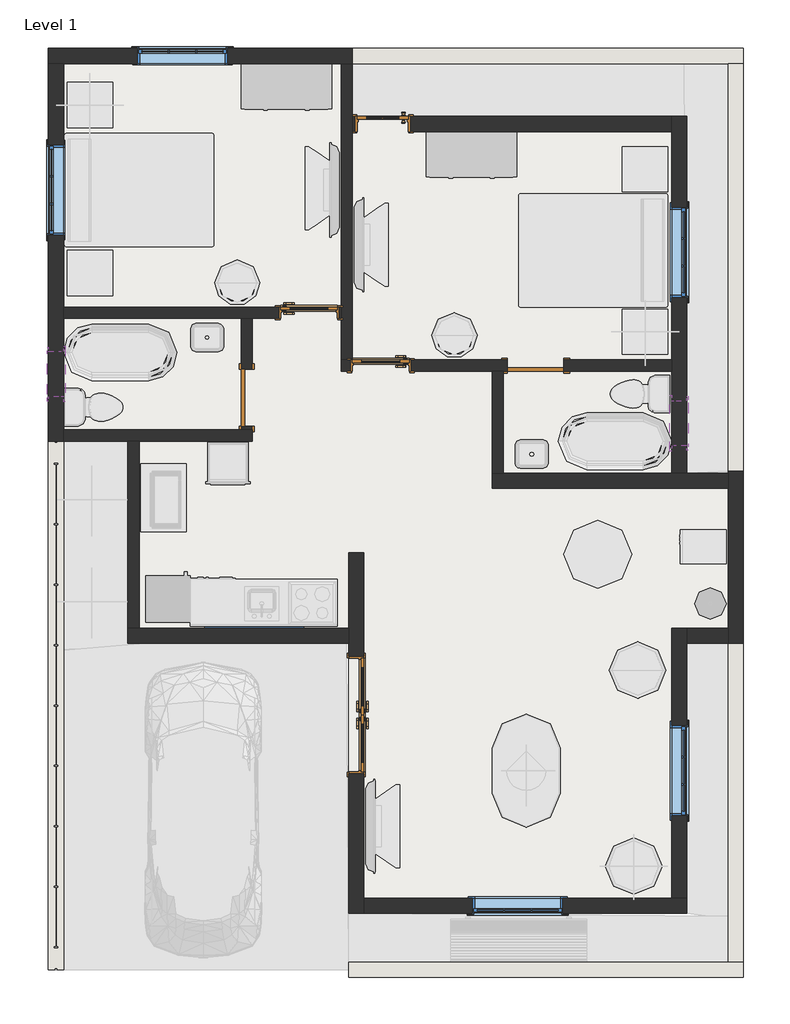
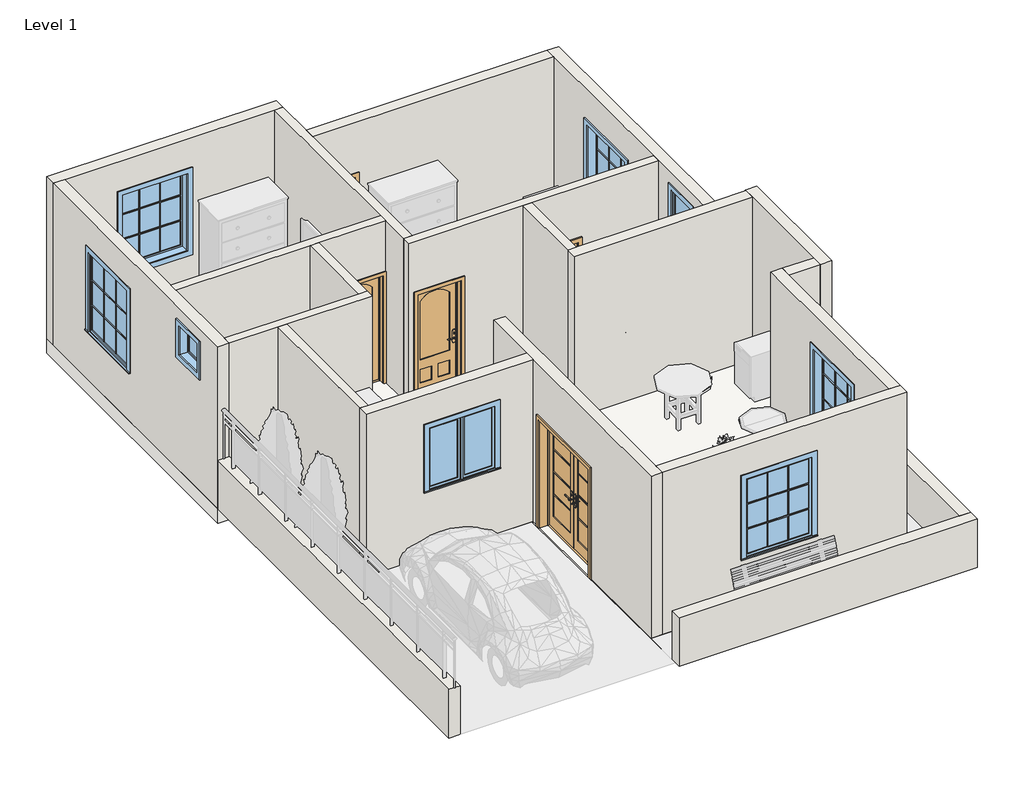
# One storey, part 1 of 2: 23 walls, 8 windows, 6 doors, 1 slab.
"""IFC4 building model written with IfcOpenShell, lengths in millimetres."""

from ifc_helpers import new_model, si_unit, frame, origin, origin_with_axes, place, context, project, spatial, polyline, outline, extrude, faceted_brep, transform, mapped, element, save
from components import door_4b146b56, door_14b9be53, door_b03bd389, door_30d62acf, door_059fdd7e, door_255cab33, window_cfa1ffdd, window_0862ab64, window_e41d21a6

model = new_model("IFC4")

# Units and contexts
model_context = context("Model", 3, world=origin())
ifc_project = project(units=[si_unit("LENGTHUNIT", "METRE", prefix="MILLI")], contexts=[model_context])

# Site, building, storey
site = spatial("IfcSite", under=ifc_project)
building = spatial("IfcBuilding", under=site)
storey = spatial("IfcBuildingStorey", under=building, Name="Level 1", Elevation=0.0)

# Doors
placement = place(None, origin())
door_shape = door_4b146b56(model_context)
element("IfcDoor", 1, ObjectType="30\" x 80\"", at=placement, inside=storey, context=model_context, shape_type="MappedRepresentation", body=[
    mapped(door_shape, transform((-6599.082173, 11998.2176639, 0.0), x_axis=(-1.0, 0.0, 0.0), y_axis=(0.0, -1.0, 0.0), z_axis=(0.0, 0.0, 1.0))),
])
door_2_shape = door_14b9be53(model_context)
element("IfcDoor", 2, ObjectType="30\" x 80\"", at=placement, inside=storey, context=model_context, shape_type="MappedRepresentation", body=[
    mapped(door_2_shape, transform((-5633.882173, 11287.0176639, 0.0), x_axis=(1.0, 0.0, 0.0), y_axis=(0.0, 1.0, 0.0), z_axis=(0.0, 0.0, 1.0))),
])
door_3_shape = door_b03bd389(model_context)
element("IfcDoor", 3, ObjectType="Door-Exterior-Double-Full Glass-Wood_Clad : 60\" x 80\"", at=placement, inside=storey, context=model_context, shape_type="MappedRepresentation", body=[
    mapped(door_3_shape, transform((-5960.907173, 6584.8426639, 0.0), x_axis=(0.0, -1.0, 0.0), y_axis=(1.0, 0.0, 0.0), z_axis=(0.0, 0.0, 1.0))),
])
door_4_shape = door_30d62acf(model_context)
element("IfcDoor", 4, ObjectType="Door-Interior-Single-Full Glass-Wood : 27\" x 80\"", at=placement, inside=storey, context=model_context, shape_type="MappedRepresentation", body=[
    mapped(door_4_shape, transform((-5608.482173, 14538.2176639, 0.0), x_axis=(-1.0, 0.0, 0.0), y_axis=(0.0, -1.0, 0.0), z_axis=(0.0, 0.0, 1.0))),
])
door_5_shape = door_059fdd7e(model_context)
element("IfcDoor", 5, ObjectType="Single-Flush : 30\" x 80\"", at=placement, inside=storey, context=model_context, shape_type="MappedRepresentation", body=[
    mapped(door_5_shape, transform((-3551.082173, 11283.8426639, 0.0), x_axis=(-1.0, 0.0, 0.0), y_axis=(0.0, -1.0, 0.0), z_axis=(0.0, 0.0, 1.0))),
])
door_6_shape = door_255cab33(model_context)
element("IfcDoor", 6, ObjectType="Single-Flush : 30\" x 80\"", at=placement, inside=storey, context=model_context, shape_type="MappedRepresentation", body=[
    mapped(door_6_shape, transform((-7437.282173, 10852.0426639, 0.0), x_axis=(0.0, -1.0, 0.0), y_axis=(1.0, 0.0, 0.0), z_axis=(0.0, 0.0, 1.0))),
])

# Slab
element("IfcSlab", 7, ObjectType="Wood Joist 10\" - Ceramic Tile", at=placement, inside=storey, context=model_context, shape_type="SweptSolid", body=[
    extrude(outline(polyline([(-6014.882173, 15551.0426639), (-6014.882173, 14636.6426639), (-1519.082173, 14636.6426639), (-1519.082173, 9836.0426639), (-757.082173, 9836.0426639), (-757.082173, 7550.0426639), (-1519.082173, 7550.0426639), (-1519.082173, 3917.8426639), (-6065.682173, 3917.8426639), (-6065.682173, 7550.0426639), (-9037.482173, 7550.0426639), (-9037.482173, 10267.8426639), (-10104.282173, 10267.8426639), (-10104.282173, 15551.0426639), (-6014.882173, 15551.0426639)])), frame((0.0, 0.0, -273.05), z_axis=(0.0, 0.0, 1.0), x_axis=(1.0, 0.0, 0.0)), (0.0, 0.0, 1.0), 273.05),
])

# Walls
element("IfcWall", 8, ObjectType="Generic - 8\"", at=placement, inside=storey, context=model_context, shape_type="Brep", body=[
    faceted_brep([(-1722.282173, 14636.6426639, 0.0), (-1722.282173, 14433.4426639, 0.0), (-1722.282173, 11360.0426639, 0.0), (-1722.282173, 11207.6426639, 0.0), (-1722.282173, 9836.0426639, 0.0), (-1722.282173, 9836.0426639, 3048.0), (-1722.282173, 11207.6426639, 3048.0), (-1722.282173, 11360.0426639, 3048.0), (-1722.282173, 14433.4426639, 3048.0), (-1722.282173, 14636.6426639, 3048.0), (-1722.282173, 12198.2426639, 2438.4), (-1722.282173, 12198.2426639, 914.4), (-1722.282173, 13417.4426639, 914.4), (-1722.282173, 13417.4426639, 2438.4), (-1722.282173, 10813.9426639, 2768.6), (-1722.282173, 10204.3426639, 2768.6), (-1722.282173, 10204.3426639, 2159.0), (-1722.282173, 10813.9426639, 2159.0), (-1519.082173, 14636.6426639, 0.0), (-1519.082173, 14636.6426639, 3048.0), (-1519.082173, 9836.0426639, 3048.0), (-1519.082173, 9836.0426639, 0.0), (-1519.082173, 12198.2426639, 2438.4), (-1519.082173, 13417.4426639, 2438.4), (-1519.082173, 13417.4426639, 914.4), (-1519.082173, 12198.2426639, 914.4), (-1519.082173, 10813.9426639, 2768.6), (-1519.082173, 10813.9426639, 2159.0), (-1519.082173, 10204.3426639, 2159.0), (-1519.082173, 10204.3426639, 2768.6)], [[[0, 1, 2, 3, 4, 5, 6, 7, 8, 9], [10, 11, 12, 13], [14, 15, 16, 17]], [[18, 19, 20, 21], [22, 23, 24, 25], [26, 27, 28, 29]], [[4, 3, 2, 1, 0, 18, 21]], [[9, 8, 7, 6, 5, 20, 19]], [[5, 4, 21, 20]], [[0, 9, 19, 18]], [[11, 10, 22, 25]], [[12, 11, 25, 24]], [[13, 12, 24, 23]], [[10, 13, 23, 22]], [[27, 26, 14, 17]], [[28, 27, 17, 16]], [[29, 28, 16, 15]], [[26, 29, 15, 14]]]),
])
element("IfcWall", 9, ObjectType="Generic - 8\"", at=placement, inside=storey, context=model_context, shape_type="Brep", body=[
    faceted_brep([(-5862.482173, 3917.8426639, 0.0), (-1519.082173, 3917.8426639, 0.0), (-1519.082173, 3917.8426639, 3048.0), (-5862.482173, 3917.8426639, 3048.0), (-4401.982173, 3917.8426639, 2438.4), (-3182.782173, 3917.8426639, 2438.4), (-3182.782173, 3917.8426639, 914.4), (-4401.982173, 3917.8426639, 914.4), (-5862.482173, 4121.0426639, 0.0), (-5862.482173, 4121.0426639, 3048.0), (-1722.282173, 4121.0426639, 3048.0), (-1519.082173, 4121.0426639, 3048.0), (-1519.082173, 4121.0426639, 0.0), (-1722.282173, 4121.0426639, 0.0), (-4401.982173, 4121.0426639, 2438.4), (-4401.982173, 4121.0426639, 914.4), (-3182.782173, 4121.0426639, 914.4), (-3182.782173, 4121.0426639, 2438.4)], [[[0, 1, 2, 3], [4, 5, 6, 7]], [[8, 9, 10, 11, 12, 13], [14, 15, 16, 17]], [[1, 0, 8, 13, 12]], [[2, 1, 12, 11]], [[3, 2, 11, 10, 9]], [[0, 3, 9, 8]], [[15, 14, 4, 7]], [[16, 15, 7, 6]], [[17, 16, 6, 5]], [[14, 17, 5, 4]]]),
])
element("IfcWall", 10, ObjectType="Generic - 8\"", at=placement, inside=storey, context=model_context, shape_type="Brep", body=[
    faceted_brep([(-1519.082173, 4121.0426639, 0.0), (-1519.082173, 7550.0426639, 0.0), (-1519.082173, 7753.2426639, 0.0), (-1519.082173, 7753.2426639, 3048.0), (-1519.082173, 7550.0426639, 3048.0), (-1519.082173, 4121.0426639, 3048.0), (-1519.082173, 5225.9426639, 2438.4), (-1519.082173, 6445.1426639, 2438.4), (-1519.082173, 6445.1426639, 914.4), (-1519.082173, 5225.9426639, 914.4), (-1722.282173, 4121.0426639, 0.0), (-1722.282173, 4121.0426639, 3048.0), (-1722.282173, 7753.2426639, 3048.0), (-1722.282173, 7753.2426639, 0.0), (-1722.282173, 5225.9426639, 2438.4), (-1722.282173, 5225.9426639, 914.4), (-1722.282173, 6445.1426639, 914.4), (-1722.282173, 6445.1426639, 2438.4)], [[[0, 1, 2, 3, 4, 5], [6, 7, 8, 9]], [[10, 11, 12, 13], [14, 15, 16, 17]], [[2, 1, 0, 10, 13]], [[5, 4, 3, 12, 11]], [[0, 5, 11, 10]], [[3, 2, 13, 12]], [[15, 14, 6, 9]], [[16, 15, 9, 8]], [[17, 16, 8, 7]], [[14, 17, 7, 6]]]),
])
element("IfcWall", 11, ObjectType="Generic - 8\"", at=placement, inside=storey, context=model_context, shape_type="SweptSolid", body=[
    extrude(outline(polyline([(-1519.082173, 7753.2426639), (-960.282173, 7753.2426639), (-960.282173, 7550.0426639), (-1519.082173, 7550.0426639), (-1519.082173, 7753.2426639)])), origin_with_axes(), (0.0, 0.0, 1.0), 3048.0),
])
element("IfcWall", 12, ObjectType="Generic - 8\"", at=placement, inside=storey, context=model_context, shape_type="Brep", body=[
    faceted_brep([(-6065.682173, 3917.8426639, 3048.0), (-6065.682173, 7550.0426639, 3048.0), (-6065.682173, 7753.2426639, 3048.0), (-6065.682173, 8769.2426639, 3048.0), (-6065.682173, 8769.2426639, 0.0), (-6065.682173, 7753.2426639, 0.0), (-6065.682173, 7550.0426639, 0.0), (-6065.682173, 7372.2426639, 0.0), (-6065.682173, 7372.2426639, 2057.4), (-6065.682173, 5797.4426639, 2057.4), (-6065.682173, 5797.4426639, 0.0), (-6065.682173, 3917.8426639, 0.0), (-5862.482173, 8769.2426639, 3048.0), (-5862.482173, 4121.0426639, 3048.0), (-5862.482173, 3917.8426639, 3048.0), (-5862.482173, 3917.8426639, 0.0), (-5862.482173, 4121.0426639, 0.0), (-5862.482173, 5797.4426639, 0.0), (-5862.482173, 5797.4426639, 2057.4), (-5862.482173, 7372.2426639, 2057.4), (-5862.482173, 7372.2426639, 0.0), (-5862.482173, 8769.2426639, 0.0)], [[[0, 1, 2, 3, 4, 5, 6, 7, 8, 9, 10, 11]], [[12, 13, 14, 15, 16, 17, 18, 19, 20, 21]], [[4, 21, 20, 7, 6, 5]], [[15, 11, 10, 17, 16]], [[3, 2, 1, 0, 14, 13, 12]], [[4, 3, 12, 21]], [[0, 11, 15, 14]], [[9, 18, 17, 10]], [[18, 9, 8, 19]], [[19, 8, 7, 20]]]),
])
element("IfcWall", 13, ObjectType="Generic - 8\"", at=placement, inside=storey, context=model_context, shape_type="Brep", body=[
    faceted_brep([(-4135.282173, 9632.8426639, 0.0), (-960.282173, 9632.8426639, 0.0), (-960.282173, 9632.8426639, 3048.0), (-4135.282173, 9632.8426639, 3048.0), (-4135.282173, 9836.0426639, 0.0), (-4135.282173, 9836.0426639, 3048.0), (-3982.882173, 9836.0426639, 3048.0), (-1722.282173, 9836.0426639, 3048.0), (-1519.082173, 9836.0426639, 3048.0), (-960.282173, 9836.0426639, 3048.0), (-960.282173, 9836.0426639, 0.0), (-1519.082173, 9836.0426639, 0.0), (-1722.282173, 9836.0426639, 0.0), (-3982.882173, 9836.0426639, 0.0)], [[[0, 1, 2, 3]], [[4, 5, 6, 7, 8, 9, 10, 11, 12, 13]], [[1, 0, 4, 13, 12, 11, 10]], [[3, 2, 9, 8, 7, 6, 5]], [[2, 1, 10, 9]], [[0, 3, 5, 4]]]),
])
element("IfcWall", 14, ObjectType="Generic - 8\"", at=placement, inside=storey, context=model_context, shape_type="SweptSolid", body=[
    extrude(outline(polyline([(3048.0, -1722.282173), (3048.0, -6014.882173), (0.0, -6014.882173), (0.0, -5976.782173), (2057.4, -5976.782173), (2057.4, -5240.182173), (0.0, -5240.182173), (0.0, -1722.282173), (3048.0, -1722.282173)])), frame((0.0, 14433.4426639, 0.0), z_axis=(0.0, 1.0, 0.0), x_axis=(0.0, 0.0, 1.0)), (0.0, 0.0, 1.0), 203.2),
])
element("IfcWall", 15, ObjectType="Generic - 8\"", at=placement, inside=storey, context=model_context, shape_type="Brep", body=[
    faceted_brep([(-9037.482173, 7550.0426639, 0.0), (-6065.682173, 7550.0426639, 0.0), (-6065.682173, 7550.0426639, 3048.0), (-9037.482173, 7550.0426639, 3048.0), (-7945.282173, 7550.0426639, 2438.4), (-6726.082173, 7550.0426639, 2438.4), (-6726.082173, 7550.0426639, 1219.2), (-7945.282173, 7550.0426639, 1219.2), (-9037.482173, 7753.2426639, 0.0), (-9037.482173, 7753.2426639, 3048.0), (-8885.082173, 7753.2426639, 3048.0), (-6065.682173, 7753.2426639, 3048.0), (-6065.682173, 7753.2426639, 0.0), (-8885.082173, 7753.2426639, 0.0), (-7945.282173, 7753.2426639, 2438.4), (-7945.282173, 7753.2426639, 1219.2), (-6726.082173, 7753.2426639, 1219.2), (-6726.082173, 7753.2426639, 2438.4)], [[[0, 1, 2, 3], [4, 5, 6, 7]], [[8, 9, 10, 11, 12, 13], [14, 15, 16, 17]], [[1, 0, 8, 13, 12]], [[3, 2, 11, 10, 9]], [[0, 3, 9, 8]], [[2, 1, 12, 11]], [[15, 14, 4, 7]], [[16, 15, 7, 6]], [[17, 16, 6, 5]], [[14, 17, 5, 4]]]),
])
element("IfcWall", 16, ObjectType="INNER WALL", at=placement, inside=storey, context=model_context, shape_type="Brep", body=[
    faceted_brep([(-6167.282173, 11360.0426639, 3048.0), (-6014.882173, 11360.0426639, 3048.0), (-1722.282173, 11360.0426639, 3048.0), (-1722.282173, 11360.0426639, 0.0), (-3170.082173, 11360.0426639, 0.0), (-3170.082173, 11360.0426639, 2032.0), (-3932.082173, 11360.0426639, 2032.0), (-3932.082173, 11360.0426639, 0.0), (-5227.482173, 11360.0426639, 0.0), (-5227.482173, 11360.0426639, 2057.4), (-6040.282173, 11360.0426639, 2057.4), (-6040.282173, 11360.0426639, 0.0), (-6167.282173, 11360.0426639, 0.0), (-1722.282173, 11207.6426639, 3048.0), (-3982.882173, 11207.6426639, 3048.0), (-4135.282173, 11207.6426639, 3048.0), (-6167.282173, 11207.6426639, 3048.0), (-6167.282173, 11207.6426639, 0.0), (-6040.282173, 11207.6426639, 0.0), (-6040.282173, 11207.6426639, 2057.4), (-5227.482173, 11207.6426639, 2057.4), (-5227.482173, 11207.6426639, 0.0), (-4135.282173, 11207.6426639, 0.0), (-3982.882173, 11207.6426639, 0.0), (-3932.082173, 11207.6426639, 0.0), (-3932.082173, 11207.6426639, 2032.0), (-3170.082173, 11207.6426639, 2032.0), (-3170.082173, 11207.6426639, 0.0), (-1722.282173, 11207.6426639, 0.0)], [[[0, 1, 2, 3, 4, 5, 6, 7, 8, 9, 10, 11, 12]], [[13, 14, 15, 16, 17, 18, 19, 20, 21, 22, 23, 24, 25, 26, 27, 28]], [[3, 28, 27, 4]], [[17, 12, 11, 18]], [[7, 24, 23, 22, 21, 8]], [[2, 1, 0, 16, 15, 14, 13]], [[3, 2, 13, 28]], [[0, 12, 17, 16]], [[25, 24, 7, 6]], [[26, 25, 6, 5]], [[27, 26, 5, 4]], [[20, 9, 8, 21]], [[9, 20, 19, 10]], [[10, 19, 18, 11]]]),
])
element("IfcWall", 17, ObjectType="INNER WALL", at=placement, inside=storey, context=model_context, shape_type="SweptSolid", body=[
    extrude(outline(polyline([(-3982.882173, 11207.6426639), (-3982.882173, 9836.0426639), (-4135.282173, 9836.0426639), (-4135.282173, 11207.6426639), (-3982.882173, 11207.6426639)])), origin_with_axes(), (0.0, 0.0, 1.0), 3048.0),
])
element("IfcWall", 18, ObjectType="INNER WALL", at=placement, inside=storey, context=model_context, shape_type="SweptSolid", body=[
    extrude(outline(polyline([(-8885.082173, 10267.8426639), (-8885.082173, 7753.2426639), (-9037.482173, 7753.2426639), (-9037.482173, 10267.8426639), (-8885.082173, 10267.8426639)])), origin_with_axes(), (0.0, 0.0, 1.0), 3048.0),
])
element("IfcWall", 19, ObjectType="INNER WALL", at=placement, inside=storey, context=model_context, shape_type="Brep", body=[
    faceted_brep([(-7361.082173, 10420.2426639, 0.0), (-7513.482173, 10420.2426639, 0.0), (-9901.082173, 10420.2426639, 0.0), (-9901.082173, 10420.2426639, 3048.0), (-7513.482173, 10420.2426639, 3048.0), (-7361.082173, 10420.2426639, 3048.0), (-7361.082173, 10267.8426639, 0.0), (-7361.082173, 10267.8426639, 3048.0), (-8885.082173, 10267.8426639, 3048.0), (-9037.482173, 10267.8426639, 3048.0), (-9901.082173, 10267.8426639, 3048.0), (-9901.082173, 10267.8426639, 0.0), (-9037.482173, 10267.8426639, 0.0), (-8885.082173, 10267.8426639, 0.0)], [[[0, 1, 2, 3, 4, 5]], [[6, 7, 8, 9, 10, 11, 12, 13]], [[2, 1, 0, 6, 13, 12, 11]], [[5, 4, 3, 10, 9, 8, 7]], [[0, 5, 7, 6]], [[2, 11, 10, 3]]]),
])
element("IfcWall", 20, ObjectType="INNER WALL", at=placement, inside=storey, context=model_context, shape_type="SweptSolid", body=[
    extrude(outline(polyline([(10471.0426639, 2032.0), (10471.0426639, 0.0), (10420.2426639, 0.0), (10420.2426639, 3048.0), (11918.8426639, 3048.0), (11918.8426639, 0.0), (11233.0426639, 0.0), (11233.0426639, 2032.0), (10471.0426639, 2032.0)])), frame((-7513.482173, 0.0, 0.0), z_axis=(1.0, 0.0, 0.0), x_axis=(0.0, 1.0, 0.0)), (0.0, 0.0, 1.0), 152.4),
])
element("IfcWall", 21, ObjectType="INNER WALL", at=placement, inside=storey, context=model_context, shape_type="Brep", body=[
    faceted_brep([(-6167.282173, 15347.8426639, 3048.0), (-6167.282173, 15347.8426639, 0.0), (-6167.282173, 12071.2426639, 0.0), (-6167.282173, 11918.8426639, 0.0), (-6167.282173, 11360.0426639, 0.0), (-6167.282173, 11360.0426639, 3048.0), (-6167.282173, 11918.8426639, 3048.0), (-6167.282173, 12071.2426639, 3048.0), (-6014.882173, 15347.8426639, 0.0), (-6014.882173, 15347.8426639, 3048.0), (-6014.882173, 14636.6426639, 3048.0), (-6014.882173, 14433.4426639, 3048.0), (-6014.882173, 11360.0426639, 3048.0), (-6014.882173, 11360.0426639, 0.0), (-6014.882173, 14433.4426639, 0.0), (-6014.882173, 14636.6426639, 0.0), (-6040.282173, 11360.0426639, 0.0)], [[[0, 1, 2, 3, 4, 5, 6, 7]], [[8, 9, 10, 11, 12, 13, 14, 15]], [[4, 3, 2, 1, 8, 15, 14, 13, 16]], [[0, 7, 6, 5, 12, 11, 10, 9]], [[5, 4, 16, 13, 12]], [[0, 9, 8, 1]]]),
])
element("IfcWall", 22, ObjectType="INNER WALL", at=placement, inside=storey, context=model_context, shape_type="Brep", body=[
    faceted_brep([(-9901.082173, 12071.2426639, 3048.0), (-6167.282173, 12071.2426639, 3048.0), (-6167.282173, 12071.2426639, 0.0), (-6192.682173, 12071.2426639, 0.0), (-6192.682173, 12071.2426639, 2057.4), (-7005.482173, 12071.2426639, 2057.4), (-7005.482173, 12071.2426639, 0.0), (-9901.082173, 12071.2426639, 0.0), (-6167.282173, 11918.8426639, 3048.0), (-7361.082173, 11918.8426639, 3048.0), (-7513.482173, 11918.8426639, 3048.0), (-9901.082173, 11918.8426639, 3048.0), (-9901.082173, 11918.8426639, 0.0), (-7513.482173, 11918.8426639, 0.0), (-7361.082173, 11918.8426639, 0.0), (-7005.482173, 11918.8426639, 0.0), (-7005.482173, 11918.8426639, 2057.4), (-6192.682173, 11918.8426639, 2057.4), (-6192.682173, 11918.8426639, 0.0), (-6167.282173, 11918.8426639, 0.0)], [[[0, 1, 2, 3, 4, 5, 6, 7]], [[8, 9, 10, 11, 12, 13, 14, 15, 16, 17, 18, 19]], [[2, 19, 18, 3]], [[12, 7, 6, 15, 14, 13]], [[1, 0, 11, 10, 9, 8]], [[2, 1, 8, 19]], [[0, 7, 12, 11]], [[5, 16, 15, 6]], [[16, 5, 4, 17]], [[17, 4, 3, 18]]]),
])
element("IfcWall", 23, ObjectType="OUTER WALL", at=placement, inside=storey, context=model_context, shape_type="Brep", body=[
    faceted_brep([(-10104.282173, 15347.8426639, 0.0), (-9901.082173, 15347.8426639, 0.0), (-6167.282173, 15347.8426639, 0.0), (-6014.882173, 15347.8426639, 0.0), (-6014.882173, 15347.8426639, 914.4), (-6014.882173, 15347.8426639, 3048.0), (-6167.282173, 15347.8426639, 3048.0), (-9901.082173, 15347.8426639, 3048.0), (-10104.282173, 15347.8426639, 3048.0), (-7691.282173, 15347.8426639, 2438.4), (-7691.282173, 15347.8426639, 914.4), (-8910.482173, 15347.8426639, 914.4), (-8910.482173, 15347.8426639, 2438.4), (-10104.282173, 15551.0426639, 0.0), (-10104.282173, 15551.0426639, 3048.0), (-6014.882173, 15551.0426639, 3048.0), (-6014.882173, 15551.0426639, 914.4), (-6014.882173, 15551.0426639, 0.0), (-7691.282173, 15551.0426639, 2438.4), (-8910.482173, 15551.0426639, 2438.4), (-8910.482173, 15551.0426639, 914.4), (-7691.282173, 15551.0426639, 914.4)], [[[0, 1, 2, 3, 4, 5, 6, 7, 8], [9, 10, 11, 12]], [[13, 14, 15, 16, 17], [18, 19, 20, 21]], [[3, 2, 1, 0, 13, 17]], [[8, 7, 6, 5, 15, 14]], [[0, 8, 14, 13]], [[3, 17, 16, 15, 5, 4]], [[10, 9, 18, 21]], [[11, 10, 21, 20]], [[12, 11, 20, 19]], [[9, 12, 19, 18]]]),
])
element("IfcWall", 24, ObjectType="OUTER WALL", at=placement, inside=storey, context=model_context, shape_type="SweptSolid", body=[
    extrude(outline(polyline([(-960.282173, 9861.4426639), (-960.282173, 15347.8426639), (-757.082173, 15347.8426639), (-757.082173, 9861.4426639), (-960.282173, 9861.4426639)])), origin_with_axes(), (0.0, 0.0, 1.0), 914.4),
])
element("IfcWall", 25, ObjectType="OUTER WALL", at=placement, inside=storey, context=model_context, shape_type="Brep", body=[
    faceted_brep([(-10104.282173, 15347.8426639, 0.0), (-10104.282173, 10267.8426639, 0.0), (-10104.282173, 10267.8426639, 914.4), (-10104.282173, 10267.8426639, 3048.0), (-10104.282173, 15347.8426639, 3048.0), (-10104.282173, 14255.6426639, 2438.4), (-10104.282173, 13036.4426639, 2438.4), (-10104.282173, 13036.4426639, 914.4), (-10104.282173, 14255.6426639, 914.4), (-10104.282173, 10864.7426639, 2768.6), (-10104.282173, 10864.7426639, 2159.0), (-10104.282173, 11474.3426639, 2159.0), (-10104.282173, 11474.3426639, 2768.6), (-9901.082173, 15347.8426639, 0.0), (-9901.082173, 15347.8426639, 3048.0), (-9901.082173, 12071.2426639, 3048.0), (-9901.082173, 11918.8426639, 3048.0), (-9901.082173, 10420.2426639, 3048.0), (-9901.082173, 10267.8426639, 3048.0), (-9901.082173, 10267.8426639, 914.4), (-9901.082173, 10267.8426639, 0.0), (-9901.082173, 10420.2426639, 0.0), (-9901.082173, 11918.8426639, 0.0), (-9901.082173, 12071.2426639, 0.0), (-9901.082173, 14255.6426639, 2438.4), (-9901.082173, 14255.6426639, 914.4), (-9901.082173, 13036.4426639, 914.4), (-9901.082173, 13036.4426639, 2438.4), (-9901.082173, 10864.7426639, 2768.6), (-9901.082173, 11474.3426639, 2768.6), (-9901.082173, 11474.3426639, 2159.0), (-9901.082173, 10864.7426639, 2159.0)], [[[0, 1, 2, 3, 4], [5, 6, 7, 8], [9, 10, 11, 12]], [[13, 14, 15, 16, 17, 18, 19, 20, 21, 22, 23], [24, 25, 26, 27], [28, 29, 30, 31]], [[1, 0, 13, 23, 22, 21, 20]], [[3, 2, 1, 20, 19, 18]], [[4, 3, 18, 17, 16, 15, 14]], [[0, 4, 14, 13]], [[25, 24, 5, 8]], [[26, 25, 8, 7]], [[27, 26, 7, 6]], [[24, 27, 6, 5]], [[10, 9, 28, 31]], [[11, 10, 31, 30]], [[12, 11, 30, 29]], [[9, 12, 29, 28]]]),
])
element("IfcWall", 26, ObjectType="OUTER WALL", at=placement, inside=storey, context=model_context, shape_type="Brep", body=[
    faceted_brep([(-6065.682173, 3054.2426639, 0.0), (-757.082173, 3054.2426639, 0.0), (-757.082173, 3054.2426639, 914.4), (-6065.682173, 3054.2426639, 914.4), (-6065.682173, 3257.4426639, 0.0), (-6065.682173, 3257.4426639, 914.4), (-960.282173, 3257.4426639, 914.4), (-757.082173, 3257.4426639, 914.4), (-757.082173, 3257.4426639, 0.0), (-960.282173, 3257.4426639, 0.0)], [[[0, 1, 2, 3]], [[4, 5, 6, 7, 8, 9]], [[1, 0, 4, 9, 8]], [[3, 2, 7, 6, 5]], [[0, 3, 5, 4]], [[2, 1, 8, 7]]]),
])
element("IfcWall", 27, ObjectType="OUTER WALL", at=placement, inside=storey, context=model_context, shape_type="SweptSolid", body=[
    extrude(outline(polyline([(-960.282173, 3257.4426639), (-960.282173, 7550.0426639), (-757.082173, 7550.0426639), (-757.082173, 3257.4426639), (-960.282173, 3257.4426639)])), origin_with_axes(), (0.0, 0.0, 1.0), 914.4),
])
element("IfcWall", 28, ObjectType="OUTER WALL", at=placement, inside=storey, context=model_context, shape_type="Brep", body=[
    faceted_brep([(-6014.882173, 15347.8426639, 0.0), (-960.282173, 15347.8426639, 0.0), (-757.082173, 15347.8426639, 0.0), (-757.082173, 15347.8426639, 914.4), (-960.282173, 15347.8426639, 914.4), (-6014.882173, 15347.8426639, 914.4), (-6014.882173, 15551.0426639, 0.0), (-6014.882173, 15551.0426639, 914.4), (-757.082173, 15551.0426639, 914.4), (-757.082173, 15551.0426639, 0.0)], [[[0, 1, 2, 3, 4, 5]], [[6, 7, 8, 9]], [[2, 1, 0, 6, 9]], [[5, 4, 3, 8, 7]], [[3, 2, 9, 8]], [[0, 5, 7, 6]]]),
])
element("IfcWall", 29, ObjectType="OUTER WALL", at=placement, inside=storey, context=model_context, shape_type="Brep", body=[
    faceted_brep([(-960.282173, 9861.4426639, 0.0), (-960.282173, 9836.0426639, 0.0), (-960.282173, 9632.8426639, 0.0), (-960.282173, 7753.2426639, 0.0), (-960.282173, 7550.0426639, 0.0), (-960.282173, 7550.0426639, 914.4), (-960.282173, 7550.0426639, 3048.0), (-960.282173, 7753.2426639, 3048.0), (-960.282173, 9632.8426639, 3048.0), (-960.282173, 9836.0426639, 3048.0), (-960.282173, 9861.4426639, 3048.0), (-960.282173, 9861.4426639, 914.4), (-757.082173, 9861.4426639, 0.0), (-757.082173, 9861.4426639, 914.4), (-757.082173, 9861.4426639, 3048.0), (-757.082173, 7550.0426639, 3048.0), (-757.082173, 7550.0426639, 914.4), (-757.082173, 7550.0426639, 0.0)], [[[0, 1, 2, 3, 4, 5, 6, 7, 8, 9, 10, 11]], [[12, 13, 14, 15, 16, 17]], [[4, 3, 2, 1, 0, 12, 17]], [[6, 5, 4, 17, 16, 15]], [[10, 9, 8, 7, 6, 15, 14]], [[0, 11, 10, 14, 13, 12]]]),
])
element("IfcWall", 30, ObjectType="OUTER WALL", at=placement, inside=storey, context=model_context, shape_type="SweptSolid", body=[
    extrude(outline(polyline([(-10104.282173, 3155.8426639), (-10104.282173, 10267.8426639), (-9901.082173, 10267.8426639), (-9901.082173, 3155.8426639), (-10104.282173, 3155.8426639)])), origin_with_axes(), (0.0, 0.0, 1.0), 914.4),
])

# Windows
window_shape = window_cfa1ffdd(model_context)
element("IfcWindow", 31, ObjectType="Casement 3x3 with Trim : 48\" x 60\"", at=placement, inside=storey, context=model_context, shape_type="MappedRepresentation", body=[
    mapped(window_shape, transform((-10002.682173, 13646.0426639, 304.8), x_axis=(0.0, 1.0, 0.0), y_axis=(-1.0, 0.0, 0.0), z_axis=(0.0, 0.0, 1.0))),
])
element("IfcWindow", 32, ObjectType="Casement 3x3 with Trim : 48\" x 60\"", at=placement, inside=storey, context=model_context, shape_type="MappedRepresentation", body=[
    mapped(window_shape, transform((-8300.882173, 15449.4426639, 304.8), x_axis=(1.0, 0.0, 0.0), y_axis=(0.0, 1.0, 0.0), z_axis=(0.0, 0.0, 1.0))),
])
element("IfcWindow", 33, ObjectType="Casement 3x3 with Trim : 48\" x 60\"", at=placement, inside=storey, context=model_context, shape_type="MappedRepresentation", body=[
    mapped(window_shape, transform((-3792.382173, 4019.4426639, 304.8), x_axis=(-1.0, 0.0, 0.0), y_axis=(0.0, -1.0, 0.0), z_axis=(0.0, 0.0, 1.0))),
])
element("IfcWindow", 34, ObjectType="Casement 3x3 with Trim : 48\" x 60\"", at=placement, inside=storey, context=model_context, shape_type="MappedRepresentation", body=[
    mapped(window_shape, transform((-1620.682173, 5835.5426639, 304.8), x_axis=(0.0, -1.0, 0.0), y_axis=(1.0, 0.0, 0.0), z_axis=(0.0, 0.0, 1.0))),
])
element("IfcWindow", 35, ObjectType="Casement 3x3 with Trim : 48\" x 60\"", at=placement, inside=storey, context=model_context, shape_type="MappedRepresentation", body=[
    mapped(window_shape, transform((-1620.682173, 12807.8426639, 304.8), x_axis=(0.0, -1.0, 0.0), y_axis=(1.0, 0.0, 0.0), z_axis=(0.0, 0.0, 1.0))),
])
window_2_shape = window_0862ab64(model_context)
element("IfcWindow", 36, ObjectType="Casement Dbl with Trim : 48\" x 48\"", at=placement, inside=storey, context=model_context, shape_type="MappedRepresentation", body=[
    mapped(window_2_shape, transform((-7335.682173, 7670.6926639, 304.8), x_axis=(-1.0, 0.0, 0.0), y_axis=(0.0, -1.0, 0.0), z_axis=(0.0, 0.0, 1.0))),
])
window_3_shape = window_e41d21a6(model_context)
element("IfcWindow", 37, ObjectType="Transom with Trim : 24\" x 24\"", at=placement, inside=storey, context=model_context, shape_type="MappedRepresentation", body=[
    mapped(window_3_shape, transform((-1620.682173, 10547.2426639, 0.0), x_axis=(0.0, 1.0, 0.0), y_axis=(-1.0, 0.0, 0.0), z_axis=(0.0, 0.0, 1.0))),
])
element("IfcWindow", 38, ObjectType="Transom with Trim : 24\" x 24\"", at=placement, inside=storey, context=model_context, shape_type="MappedRepresentation", body=[
    mapped(window_3_shape, transform((-10002.682173, 11131.4426639, 0.0), x_axis=(0.0, -1.0, 0.0), y_axis=(1.0, 0.0, 0.0), z_axis=(0.0, 0.0, 1.0))),
])

save(model, "model.ifc")

# Revit data of these elements
# Type "30\" x 80\""
#   Type Mark = "9"
#   Assembly Code = "B2030100"
#   Analytic Construction = "French door, wood frame with single glass"
#   Threshold Offset [instance default] = 0' - 0 1/2"
#   Thickness = 0' - 1 3/8"
#   Thermal Resistance (R) = 1.0696 (h·ft²·°F)/BTU
#   Swing Angle [instance default] = 90.00°
#   Stiles = 0' - 4 3/4"
#   Rough Width = 2' - 8"
#   Rough Height = 6' - 9"
#   Radius = 1' - 1.00625"
#   Lock Rail = 0' - 7 1/8"
#   Height = 6' - 8"
#   Width = 2' - 6"
#   Heat Transfer Coefficient (U) = 0.9350 BTU/(h·ft²·°F)
#   Door Offset [instance default] = 0' - 0"
#   Bottom Rail = 0' - 9 1/2"
#   Threshold [instance default] = yes
#   Function = 1
#   Exterior Trim [instance default] = yes
#   Trim Material = Cherry
#   Threshold Material = Cherry
#   Panel Material = Cherry
#   Glazing = Glass
#   Frame Material = Cherry
#   Door Handle Material = Aluminum
#   Visual Light Transmittance = 0
#   Solar Heat Gain Coefficient = 0
#   Wall Closure = (empty or 0)
#   Construction Type = (empty or 0)
# Type "Door-Exterior-Double-Full Glass-Wood_Clad : 60\" x 80\""
#   Type Mark = "8"
#   Assembly Code = "B2030100"
#   Analytic Construction = "French door, wood frame with double glass"
#   Top Rail = 0' - 4 11/16"
#   Threshold Offset [instance default] = 0' - 0 1/2"
#   Thickness = 0' - 1 3/8"
#   Thermal Resistance (R) = 1.9158 (h·ft²·°F)/BTU
#   Swing Angle [instance default] = 90.00°
#   Stiles = 0' - 4 3/4"
#   Rough Width = 5' - 2"
#   Rough Height = 6' - 9"
#   Panel Width = 2' - 6"
#   Door Offset [instance default] = 0' - 0"
#   Height = 6' - 8"
#   Width = 5' - 0"
#   Heat Transfer Coefficient (U) = 0.5220 BTU/(h·ft²·°F)
#   Bottom Rail = 0' - 9 1/8"
#   Exterior Trim [instance default] = yes
#   Threshold [instance default] = yes
#   Show Grill [instance default] = yes
#   Function = 1
#   Trim Material = Cherry
#   Threshold Material = Cherry
#   Panel Material = Cherry
#   Glazing = Glass
#   Frame Material = Cherry
#   Door Handle Material = Aluminum
#   Visual Light Transmittance = 0
#   Solar Heat Gain Coefficient = 0
#   Wall Closure = (empty or 0)
#   Construction Type = (empty or 0)
# Type "Door-Interior-Single-Full Glass-Wood : 27\" x 80\""
#   Type Mark = "10"
#   Assembly Code = "C1020300"
#   Analytic Construction = "Wood frame with single clear glass"
#   Top Rail = 0' - 4 11/16"
#   Thickness = 0' - 1 3/8"
#   Thermal Resistance (R) = 1.0102 (h·ft²·°F)/BTU
#   Swing Angle [instance default] = 90.00°
#   Stiles = 0' - 4 3/4"
#   Rough Width = 2' - 5"
#   Rough Height = 6' - 9"
#   Height = 6' - 8"
#   Width = 2' - 3"
#   Heat Transfer Coefficient (U) = 0.9900 BTU/(h·ft²·°F)
#   Bottom Rail = 0' - 9 1/8"
#   Show Grill [instance default] = yes
#   Trim Material = Cherry
#   Panel Material = Cherry
#   Frame Material = Cherry
#   Door Handle Material = Aluminum
#   Visual Light Transmittance = 0
#   Solar Heat Gain Coefficient = 0
#   Wall Closure = (empty or 0)
#   Function = (empty or 0)
# Type "Single-Flush : 30\" x 80\""
#   Type Mark = "5"
#   Construction Type Id = "MDOOR"
#   Assembly Code = "C1020"
#   Analytic Construction = "Metal"
#   Thickness = 0' - 2"
#   Heat Transfer Coefficient (U) = 0.651978 BTU/(h·ft²·°F)
#   Height = 6' - 8"
#   Trim Projection Ext = 0' - 1"
#   Trim Projection Int = 0' - 1"
#   Trim Width = 0' - 3"
#   Width = 2' - 6"
#   Define Thermal Properties by = 1
#   Door Material = Door - Panel
#   Frame Material = Door - Frame
#   Visual Light Transmittance = 0
#   Solar Heat Gain Coefficient = 0
#   Function = (empty or 0)
#   Wall Closure = (empty or 0)
# Type "Wood Joist 10\" - Ceramic Tile"
#   Assembly Code = "B1010"
#   Function = 0
#   Layers, outside or top first: 0' - 0 1/4" "Tile, Mosaic, Gray" (function 5); 0' - 0 1/2" "Concrete, Cast-in-Place gray" (function 4); 0' - 0 3/4" "Plywood, Sheathing" (function 1); 0' - 9 1/4" "Structure, Wood Joist/Rafter Layer" (function 1)
# Type "Generic - 8\""
#   Assembly Code = "B2010"
#   Layers, outside or top first: 0' - 8" "Brick, Common" (function 1)
# Type "INNER WALL"
#   Assembly Code = "B2010"
#   Layers, outside or top first: 0' - 6" "Brick, Common" (function 1)
# Type "OUTER WALL"
#   Assembly Code = "B2010"
#   Layers, outside or top first: 0' - 8" "Brick, Soldier Course" (function 1)
# Type "Casement 3x3 with Trim : 48\" x 60\""
#   Type Mark = "11"
#   Construction Type Id = "GSP4R"
#   Assembly Code = "B2020100"
#   Analytic Construction = "1/8 in Pilkington single glazing"
#   Visual Light Transmittance = 0.9
#   Solar Heat Gain Coefficient = 0.78
#   Heat Transfer Coefficient (U) = 0.6496 BTU/(h·ft²·°F)
#   Height = 5' - 0"
#   Default Sill Height = 2' - 0"
#   Trim Projection - Ext. = 0' - 0 1/2"
#   Trim Projection - Int. = 0' - 0 3/4"
#   Trim Width - Exterior = 0' - 3 1/2"
#   Trim Width - Interior = 0' - 3 1/2"
#   Width = 4' - 0"
#   Window Inset = 0' - 0 3/4"
#   Define Thermal Properties by = 1
#   Glass Pane Material = Glass
#   Sash Material = Sash
#   Trim Exterior Material = Trim
#   Trim Interior Material = Trim
#   Wall Closure = (empty or 0)
# Type "Casement Dbl with Trim : 48\" x 48\""
#   Type Mark = "13"
#   Construction Type Id = "GSP4R"
#   Assembly Code = "B2020100"
#   Analytic Construction = "1/8 in Pilkington single glazing"
#   Visual Light Transmittance = 0.9
#   Solar Heat Gain Coefficient = 0.78
#   Heat Transfer Coefficient (U) = 0.6496 BTU/(h·ft²·°F)
#   Height = 4' - 0"
#   Default Sill Height = 3' - 0"
#   Trim Projection - Ext. = 0' - 0 1/2"
#   Trim Projection - Int. = 0' - 0 3/4"
#   Trim Width - Exterior = 0' - 3 1/2"
#   Trim Width - Interior = 0' - 3 1/2"
#   Width = 4' - 0"
#   Window Inset = 0' - 0 3/4"
#   Define Thermal Properties by = 1
#   Glass Pane Material = Glass
#   Sash Material = Sash
#   Trim Exterior Material = Trim
#   Trim Interior Material = Trim
#   Wall Closure = (empty or 0)
# Type "Transom with Trim : 24\" x 24\""
#   Type Mark = "16"
#   Construction Type Id = "GSP4R"
#   Assembly Code = "B2020100"
#   Analytic Construction = "1/8 in Pilkington single glazing"
#   Visual Light Transmittance = 0.9
#   Solar Heat Gain Coefficient = 0.78
#   Heat Transfer Coefficient (U) = 0.6496 BTU/(h·ft²·°F)
#   Height = 2' - 0"
#   Default Sill Height = 7' - 1"
#   Trim Projection - Ext. = 0' - 0 1/2"
#   Trim Projection - Int. = 0' - 0 3/4"
#   Trim Width - Exterior = 0' - 3 1/2"
#   Trim Width - Interior = 0' - 3 1/2"
#   Width = 2' - 0"
#   Window Inset = 0' - 0 3/4"
#   Define Thermal Properties by = 1
#   Glass Pane Material = Glass
#   Sash Material = Sash
#   Trim Exterior Material = Trim
#   Trim Interior Material = Trim
#   Wall Closure = (empty or 0)
# Elements 1, 2 (IfcDoor, "30\" x 80\"")
#   Threshold Offset = 0' - 0 1/2"
#   Swing Angle = 90.00°
#   Door Offset = 0' - 0"
#   Threshold = yes
#   Exterior Trim = yes
#   Phase Created = New Construction
#   Materials on its faces: "Cherry", "Aluminum", "Glass"
# Element 3 (IfcDoor, "Door-Exterior-Double-Full Glass-Wood_Clad : 60\" x 80\"")
#   Threshold Offset = 0' - 0 1/2"
#   Swing Angle = 90.00°
#   Door Offset = 0' - 0"
#   Threshold = yes
#   Show Grill = yes
#   Exterior Trim = yes
#   Phase Created = New Construction
#   Materials on its faces: "Cherry", "Aluminum", "Glass"
# Element 4 (IfcDoor, "Door-Interior-Single-Full Glass-Wood : 27\" x 80\"")
#   Swing Angle = 90.00°
#   Show Grill = yes
#   Phase Created = New Construction
#   Materials on its faces: "Cherry", "Aluminum", "Glass"
# Elements 5, 6 (IfcDoor, "Single-Flush : 30\" x 80\"")
#   Phase Created = New Construction
#   Materials on its faces: "Door - Frame", "Door - Panel"
# Element 7 (IfcSlab, "Wood Joist 10\" - Ceramic Tile")
#   Height Offset From Level = 0' - 0"
#   Phase Created = New Construction
#   Materials on its faces: "Structure, Wood Joist/Rafter Layer", "Tile, Mosaic, Gray"
# Elements 8, 9, 10, 11, 12, 13, 14, 15 (IfcWall, "Generic - 8\"")
#   Top Offset = 0' - 0"
#   Base Offset = 0' - 0"
#   Unconnected Height = 10' - 0"
#   wall height = 10' - 0"
#   Phase Created = New Construction
#   Base Constraint = Level 1
#   Materials on its faces: "Brick, Common"
# Elements 16, 17, 18, 19, 20, 21, 22 (IfcWall, "INNER WALL")
#   Top Offset = 0' - 0"
#   Base Offset = 0' - 0"
#   Unconnected Height = 10' - 0"
#   wall height = 10' - 0"
#   Phase Created = New Construction
#   Base Constraint = Level 1
#   Materials on its faces: "Brick, Common"
# Element 23 (IfcWall, "OUTER WALL")
#   Top Offset = 0' - 0"
#   Base Offset = 0' - 0"
#   Unconnected Height = 10' - 0"
#   wall height = 10' - 0"
#   Phase Created = New Construction
#   Base Constraint = Level 1
#   Materials on its faces: "Brick, Soldier Course", "Brick, Common"
# Elements 24, 26, 27, 28, 30 (IfcWall, "OUTER WALL")
#   Top Offset = 0' - 0"
#   Base Offset = 0' - 0"
#   Unconnected Height = 3' - 0"
#   wall height = 3' - 0"
#   Phase Created = New Construction
#   Base Constraint = Level 1
#   Materials on its faces: "Brick, Soldier Course"
# Elements 25, 29 (IfcWall, "OUTER WALL")
#   Top Offset = 0' - 0"
#   Base Offset = 0' - 0"
#   Unconnected Height = 10' - 0"
#   wall height = 10' - 0"
#   Phase Created = New Construction
#   Base Constraint = Level 1
#   Materials on its faces: "Brick, Soldier Course"
# Element 31 (IfcWindow, "Casement 3x3 with Trim : 48\" x 60\"")
#   Mark = "4"
#   Phase Created = New Construction
#   Materials on its faces: "Sash", "Glass", "Trim"
# Element 32 (IfcWindow, "Casement 3x3 with Trim : 48\" x 60\"")
#   Mark = "5"
#   Phase Created = New Construction
#   Materials on its faces: "Sash", "Glass", "Trim"
# Element 33 (IfcWindow, "Casement 3x3 with Trim : 48\" x 60\"")
#   Mark = "1"
#   Phase Created = New Construction
#   Materials on its faces: "Sash", "Glass", "Trim"
# Element 34 (IfcWindow, "Casement 3x3 with Trim : 48\" x 60\"")
#   Mark = "2"
#   Phase Created = New Construction
#   Materials on its faces: "Sash", "Glass", "Trim"
# Element 35 (IfcWindow, "Casement 3x3 with Trim : 48\" x 60\"")
#   Mark = "3"
#   Phase Created = New Construction
#   Materials on its faces: "Sash", "Glass", "Trim"
# Element 36 (IfcWindow, "Casement Dbl with Trim : 48\" x 48\"")
#   Mark = "6"
#   Phase Created = New Construction
#   Materials on its faces: "Sash", "Trim", "Glass"
# Element 37 (IfcWindow, "Transom with Trim : 24\" x 24\"")
#   Mark = "7"
#   Phase Created = New Construction
#   Materials on its faces: "Sash", "Trim", "Glass"
# Element 38 (IfcWindow, "Transom with Trim : 24\" x 24\"")
#   Mark = "8"
#   Phase Created = New Construction
#   Materials on its faces: "Sash", "Trim", "Glass"
# Materials
#   "Cherry": class "Wood", colour RGB 226 177 128, transparency 0, Description = "Prunus Serotina", Cost = 0
#   "Glass": class "Glass", colour RGB 0 128 192, transparency 0.75, Description = "Soda Lime Glass", Cost = 0
#   "Aluminum": class "Metal", colour RGB 247 247 247, transparency 0, Description = "Aluminum 6061", Cost = 0
#   "Door - Panel": class "Wood", colour RGB 210 159 95, transparency 0
#   "Door - Frame": colour RGB 118 70 51, transparency 0
#   "Tile, Mosaic, Gray": class "Generic", colour RGB 127 127 127, transparency 0, Description = "Mosiac tile, gray", Cost = 0
#   "Concrete, Cast-in-Place gray": class "Concrete", colour RGB 192 192 192, transparency 0, Description = "Cast-in-place concrete", Cost = 0
#   "Plywood, Sheathing": class "Wood", colour RGB 212 179 113, transparency 0, Description = "Plywood, sheathing grade", Cost = 0
#   "Structure, Wood Joist/Rafter Layer": class "Wood", colour RGB 127 127 127, transparency 0, Description = "Wood framing, thermal airspace", Cost = 0
#   "Brick, Common": class "Masonry", colour RGB 170 98 104, transparency 0, Description = "Common brick", Cost = 0
#   "Brick, Soldier Course": class "Masonry", colour RGB 170 98 104, transparency 0, Description = "Common brick soldier coursed", Cost = 0
#   "Sash": class "Wood", colour RGB 224 178 126, transparency 0
#   "Trim": class "Wood", colour RGB 224 178 126, transparency 0
# Room at (-8002.334, 13991.656) mm, phase "New Construction", upper level "Level 1", upper offset 10' - 0", lower offset 0' - 0"
#   Number = "1"
#   Name = "BED ROOM"
# Room at (-8726.272, 11240.693) mm, phase "New Construction", upper level "Level 1", upper offset 10' - 0", lower offset 0' - 0"
#   Number = "2"
#   Name = "TOILET"
# Room at (-9300.018, 8774.566) mm, phase "New Construction", upper level "Level 1", upper offset 10' - 0", lower offset 0' - 0"
#   Number = "3"
#   Name = "GARDEN"
# Room at (-8002.334, 5547.746) mm, phase "New Construction", upper level "Level 1", upper offset 10' - 0", lower offset 0' - 0"
#   Number = "4"
#   Name = "PARKING"
# Room at (-3699.697, 5944.413) mm, phase "New Construction", upper level "Level 1", upper offset 10' - 0", lower offset 0' - 0"
#   Number = "5"
#   Name = "HALL/DRAWING"
# Room at (-2811.162, 8594.151) mm, phase "New Construction", upper level "Level 1", upper offset 10' - 0", lower offset 0' - 0"
#   Number = "6"
# Room at (-2811.162, 10339.487) mm, phase "New Construction", upper level "Level 1", upper offset 10' - 0", lower offset 0' - 0"
#   Number = "7"
#   Name = "TOILET"
# Room at (-3588.63, 12989.225) mm, phase "New Construction", upper level "Level 1", upper offset 10' - 0", lower offset 0' - 0"
#   Number = "8"
#   Name = "BED ROOM"
# Room at (-7514.193, 8441.751) mm, phase "New Construction", upper level "Level 1", upper offset 10' - 0", lower offset 0' - 0"
#   Number = "9"
#   Name = "KITCHEN"
